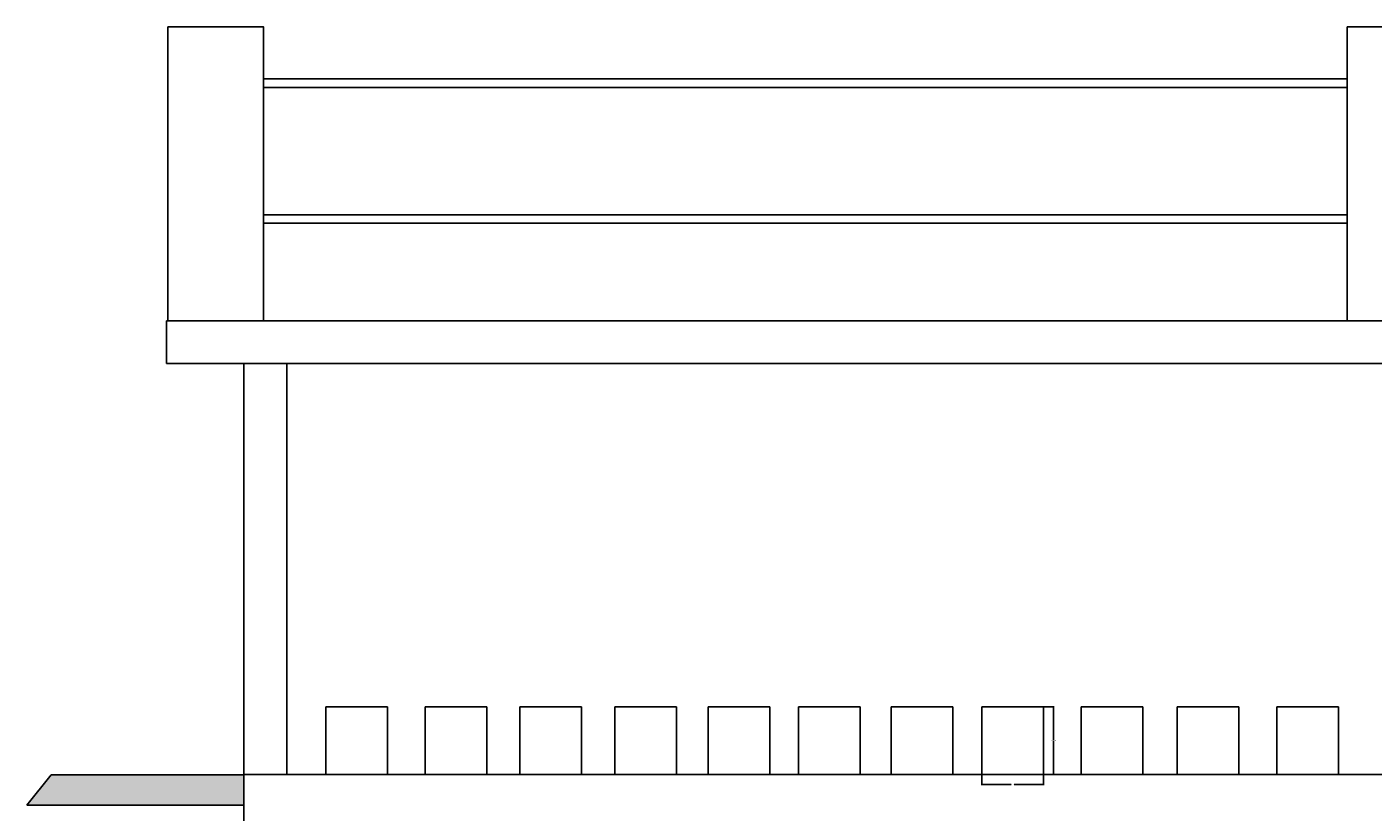
# Model space of a CAD drawing. Units: metres. Extents: x 10365 to 12529, y 3661 to 6248.
# Tile 4 of 9: x 10514 to 10987, y 5397 to 5673. Entities that reach past the tile are written whole.
import ezdxf

# ---------------------------------------------------------------- set-up
doc = ezdxf.new("R2010")
doc.units = ezdxf.units.M
doc.header["$MEASUREMENT"] = 0
for name, color, linetype, lineweight in [('A-ANNO-DIMS', 2, 'Continuous', 18), ('A-ELEV', 7, 'Continuous', 25), ('A-ELEV-PATT', 8, 'Continuous', 13)]:
    doc.layers.add(name, color=color, linetype=linetype, lineweight=lineweight)
doc.styles.get("Standard").update_dxf_attribs({"font": 'arial.ttf'})
doc.dimstyles.get("Standard").update_dxf_attribs({"dimtxt": 0.18, "dimasz": 0.18, "dimexe": 0.18, "dimexo": 0.0625, "dimgap": 0.09, "dimtad": 0, "dimtih": 1, "dimtoh": 1, "dimdec": 0, "dimzin": 0, "dimdsep": 46, "dimtxsty": 'Standard', "dimcen": 0.09, "dimadec": 0, "dimazin": 0, "dimtfac": 1, "dimtdec": 0, "dimtofl": 0, "dimtmove": 0, "dimatfit": 3, "dimfxl": 1, "dimtolj": 1, "dimtzin": 0, "dimarcsym": 0})

# ---------------------------------------------------------------- blocks, each defined once
blk = doc.blocks.new('ELEV-DENTIL')
for p, q in [((0, 0), (0, 23.79)), ((0, 23.79), (21.67, 23.79)), ((21.67, 23.79), (21.67, 0))]:
    blk.add_line(p, q)
blk = doc.blocks.new('*D33')
at = {"layer": 'A-ANNO-DIMS', "color": 0, "lineweight": -2, "transparency": 16777216}
for p, q in [((10871.7, 5433.57), (10875.39, 5433.57)), ((10875.21, 5433.39), (10875.21, 5421.85)), ((10875.21, 5409.95), (10875.21, 5421.49)), ((10871.7, 5409.77), (10875.39, 5409.77))]:
    blk.add_line(p, q, dxfattribs=at)
at = {"layer": 'A-ANNO-DIMS', "color": 0, "transparency": 16777216}
for points in [[(10875.18, 5433.39), (10875.24, 5433.39), (10875.21, 5433.57)], [(10875.18, 5409.95), (10875.24, 5409.95), (10875.21, 5409.77)]]:
    blk.add_solid(points, dxfattribs=at)
at = {"layer": 'Defpoints', "color": 0, "transparency": 16777216}
for p in [(10871.64, 5433.57), (10875.21, 5433.57), (10871.64, 5409.77)]:
    blk.add_point(p, dxfattribs=at)
at = {"layer": 'A-ANNO-DIMS', "color": 0, "transparency": 16777216, "insert": (10875.21, 5421.67), "char_height": 0.18, "attachment_point": 5}
blk.add_mtext('\\A1;DENTIL 24 TYP.', dxfattribs=at)
blk = doc.blocks.new('*D34')
at = {"layer": 'A-ANNO-DIMS', "color": 0, "lineweight": -2, "transparency": 16777216}
for p, q in [((10849.97, 5409.71), (10849.97, 5406.03)), ((10871.64, 5409.71), (10871.64, 5406.03)), ((10850.15, 5406.21), (10860.27, 5406.21)), ((10871.46, 5406.21), (10861.33, 5406.21))]:
    blk.add_line(p, q, dxfattribs=at)
at = {"layer": 'A-ANNO-DIMS', "color": 0, "transparency": 16777216}
for points in [[(10850.15, 5406.24), (10850.15, 5406.18), (10849.97, 5406.21)], [(10871.46, 5406.24), (10871.46, 5406.18), (10871.64, 5406.21)]]:
    blk.add_solid(points, dxfattribs=at)
at = {"layer": 'Defpoints', "color": 0, "transparency": 16777216}
for p in [(10849.97, 5409.77), (10871.64, 5409.77), (10871.64, 5406.21)]:
    blk.add_point(p, dxfattribs=at)
at = {"layer": 'A-ANNO-DIMS', "color": 0, "transparency": 16777216, "insert": (10860.8, 5406.21), "char_height": 0.18, "attachment_point": 5}
blk.add_mtext('\\A1;22 TYP.', dxfattribs=at)

msp = doc.modelspace()

# ---------------------------------------------------------------- hatches: boundary and pattern name
at = {"layer": 'A-ELEV-PATT'}
h = msp.add_hatch(color=256, dxfattribs=at)
h.dxf.hatch_style = 1
h.paths.add_polyline_path([(10514.47, 5399.03), (10590.74, 5399.03), (10590.74, 5409.69), (10523, 5409.69)])

# ---------------------------------------------------------------- linework, layer by layer
at = {"layer": 'A-ELEV'}
for p, q in [((10597.65, 5654.29), (10978.4, 5654.29)), ((10597.65, 5651.29), (10978.4, 5651.29)), ((10597.65, 5606.51), (10978.4, 5606.51)), ((10597.65, 5603.51), (10978.4, 5603.51)), ((11343.22, 5569.17), (10563.57, 5569.17)), ((10563.57, 5569.17), (10563.57, 5554.17)), ((10563.57, 5554.17), (10590.74, 5554.17)), ((10605.74, 5539.17), (10605.74, 5554.17)), ((10523, 5409.69), (10514.47, 5399.03)), ((10590.74, 5409.69), (10523, 5409.69)), ((10590.74, 5409.77), (11343.22, 5409.77)), ((10590.74, 5399.03), (10514.47, 5399.03))]:
    msp.add_line(p, q, dxfattribs=at)
for points in [[(10564.02, 5569.17), (10564.02, 5569.17), (10597.65, 5569.17), (10597.65, 5569.17), (10597.65, 5672.53), (10597.65, 5672.53), (10564.02, 5672.53), (10564.02, 5672.53)], [(10978.4, 5569.17), (10978.4, 5569.17), (11012.02, 5569.17), (11012.02, 5569.17), (11012.02, 5672.53), (11012.02, 5672.53), (10978.4, 5672.53), (10978.4, 5672.53)], [(11343.22, 5554.17), (11343.22, 5554.17), (10590.74, 5554.17), (10590.74, 5554.17), (10590.74, 4925.82), (10590.74, 4925.82), (11343.22, 4925.82), (11343.22, 4925.82)]]:
    msp.add_lwpolyline(points, close=True, dxfattribs=at)
msp.add_lwpolyline([(10605.74, 5539.17), (10605.74, 5409.77)], dxfattribs=at)

# ---------------------------------------------------------------- block references
for p in [(10619.47, 5409.77), (10654.44, 5409.77), (10687.7, 5409.77), (10721.05, 5409.77), (10753.86, 5409.77), (10785.57, 5409.77), (10818.12, 5409.77), (10849.97, 5409.77), (10884.84, 5409.77), (10918.68, 5409.77), (10953.66, 5409.77)]:
    msp.add_blockref('ELEV-DENTIL', p, dxfattribs=at)

# ---------------------------------------------------------------- dimensions: what is measured, and where the dimension line sits
at = {"layer": 'A-ANNO-DIMS'}
dim = msp.add_linear_dim(base=(10875.21, 5433.57), p1=(10871.64, 5409.77), p2=(10871.64, 5433.57), angle=90, text='DENTIL <> TYP.', dimstyle='Standard', override={"dimdec": 0, "dimrnd": 0, "dimzin": 0, "dimlunit": 2}, dxfattribs=at)
dim.commit()
dim.dimension.update_dxf_attribs({"geometry": '*D33', "text_midpoint": (10875.21, 5421.67)})
dim = msp.add_linear_dim(base=(10871.64, 5406.21), p1=(10849.97, 5409.77), p2=(10871.64, 5409.77), text='<> TYP.', dimstyle='Standard', override={"dimdec": 0, "dimrnd": 0, "dimzin": 0, "dimlunit": 2}, dxfattribs=at)
dim.commit()
dim.dimension.update_dxf_attribs({"geometry": '*D34', "text_midpoint": (10860.8, 5406.21)})

doc.saveas('drawing.dxf')
